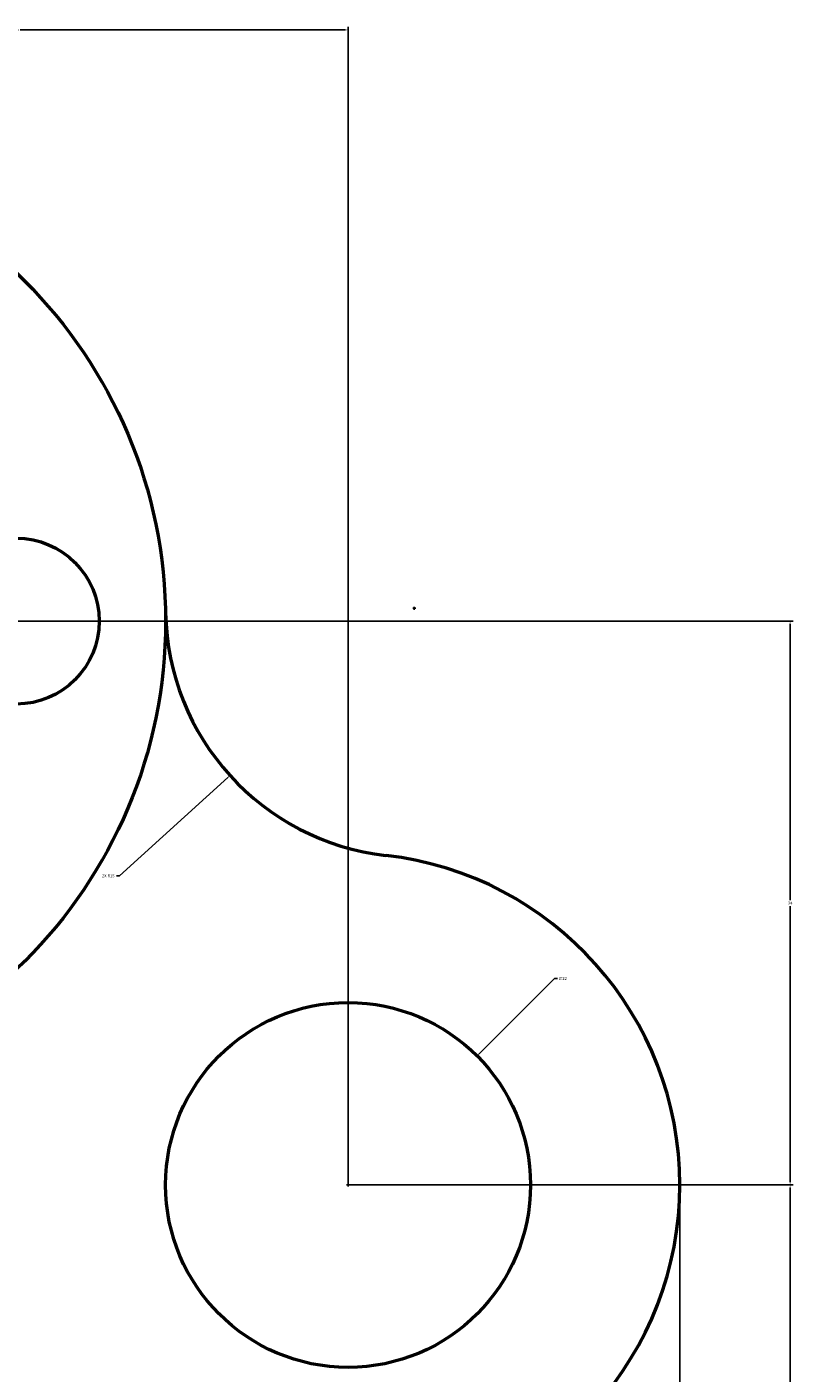
# Model space of a CAD drawing. Units: inches. Extents: x -11 to 126, y -62 to 82.
# Tile 10 of 10: x 80 to 126, y 1 to 82. Entities that reach past the tile are written whole.
import ezdxf

# ---------------------------------------------------------------- set-up
doc = ezdxf.new("R2010")
doc.units = ezdxf.units.IN
doc.header["$MEASUREMENT"] = 0
doc.layers.add('M-DIMS', color=2, linetype='Continuous', lineweight=18)
doc.layers.add('M-OUTL', color=7, linetype='Continuous', lineweight=50)
doc.styles.get("Standard").update_dxf_attribs({"font": 'arial.ttf'})
doc.dimstyles.get("Standard").update_dxf_attribs({"dimtxt": 0.18, "dimasz": 0.18, "dimexe": 0.18, "dimexo": 0.0625, "dimgap": 0.09, "dimtad": 0, "dimtih": 1, "dimtoh": 1, "dimdec": 4, "dimzin": 0, "dimdsep": 46, "dimtxsty": 'Standard', "dimcen": 0.09, "dimadec": 0, "dimazin": 0, "dimtfac": 1, "dimtdec": 4, "dimtofl": 0, "dimtmove": 0, "dimatfit": 3, "dimfxl": 1, "dimtolj": 1, "dimtzin": 0, "dimarcsym": 0})

# ---------------------------------------------------------------- blocks, each defined once
blk = doc.blocks.new('*U1')
blk.add_circle((0, 0), 5)
blk = doc.blocks.new('*U2')
at = {"layer": 'M-OUTL', "color": 0, "linetype": 'ByBlock', "lineweight": -2, "transparency": 16777216}
for p, rotation in [((73.374, 60.496), 135), ((79.232, 46.354), 90), ((73.374, 32.212), 44.99999999999998)]:
    blk.add_blockref('*U1', p, dxfattribs=dict(at, rotation=rotation))
blk = doc.blocks.new('*D5')
at = {"layer": 'Defpoints', "color": 0, "transparency": 16777216}
for p in [(119.232, 12.354), (-0.749, 11.479), (119.232, -57.296)]:
    blk.add_point(p, dxfattribs=at)
at = {"layer": 'M-DIMS', "color": 0, "lineweight": -2, "transparency": 16777216}
for p, q in [((119.232, 12.292), (119.232, -57.476)), ((-0.749, 11.416), (-0.749, -57.476)), ((-0.569, -57.296), (58.786, -57.296)), ((119.052, -57.296), (59.696, -57.296))]:
    blk.add_line(p, q, dxfattribs=at)
at = {"layer": 'M-DIMS', "color": 0, "transparency": 16777216}
for points in [[(-0.569, -57.266), (-0.569, -57.326), (-0.749, -57.296)], [(119.052, -57.266), (119.052, -57.326), (119.232, -57.296)]]:
    blk.add_solid(points, dxfattribs=at)
at = {"layer": 'M-DIMS', "color": 0, "transparency": 16777216, "insert": (59.241, -57.296), "char_height": 0.18, "attachment_point": 5}
blk.add_mtext('\\A1;119.98', dxfattribs=at)
blk = doc.blocks.new('*D8')
at = {"layer": 'Defpoints', "color": 0, "transparency": 16777216}
for p in [(99.232, 82.004), (59.232, 46.354), (99.232, 12.354)]:
    blk.add_point(p, dxfattribs=at)
at = {"layer": 'M-DIMS', "color": 0, "lineweight": -2, "transparency": 16777216}
for p, q in [((59.232, 46.417), (59.232, 82.184)), ((59.412, 82.004), (79.009, 82.004)), ((99.052, 82.004), (79.454, 82.004)), ((99.232, 12.417), (99.232, 82.184))]:
    blk.add_line(p, q, dxfattribs=at)
at = {"layer": 'M-DIMS', "color": 0, "transparency": 16777216}
for points in [[(59.412, 82.034), (59.412, 81.974), (59.232, 82.004)], [(99.052, 82.034), (99.052, 81.974), (99.232, 82.004)]]:
    blk.add_solid(points, dxfattribs=at)
at = {"layer": 'M-DIMS', "color": 0, "transparency": 16777216, "insert": (79.232, 82.004), "char_height": 0.18, "attachment_point": 5}
blk.add_mtext('\\A1;40', dxfattribs=at)
blk = doc.blocks.new('*D9')
at = {"layer": 'Defpoints', "color": 0, "transparency": 16777216}
for p in [(99.232, 12.354), (125.882, 12.354), (59.232, -21.646)]:
    blk.add_point(p, dxfattribs=at)
at = {"layer": 'M-DIMS', "color": 0, "lineweight": -2, "transparency": 16777216}
for p, q in [((99.294, 12.354), (126.062, 12.354)), ((125.882, 12.174), (125.882, -4.464)), ((125.882, -21.466), (125.882, -4.828)), ((59.294, -21.646), (126.062, -21.646))]:
    blk.add_line(p, q, dxfattribs=at)
at = {"layer": 'M-DIMS', "color": 0, "transparency": 16777216}
for points in [[(125.852, 12.174), (125.912, 12.174), (125.882, 12.354)], [(125.852, -21.466), (125.912, -21.466), (125.882, -21.646)]]:
    blk.add_solid(points, dxfattribs=at)
at = {"layer": 'M-DIMS', "color": 0, "transparency": 16777216, "insert": (125.882, -4.646), "char_height": 0.18, "attachment_point": 5}
blk.add_mtext('\\A1;34', dxfattribs=at)
blk = doc.blocks.new('*D10')
at = {"layer": 'Defpoints', "color": 0, "transparency": 16777216}
for p in [(59.232, 46.354), (125.882, 46.354), (99.232, 12.354)]:
    blk.add_point(p, dxfattribs=at)
at = {"layer": 'M-DIMS', "color": 0, "lineweight": -2, "transparency": 16777216}
for p, q in [((59.294, 46.354), (126.062, 46.354)), ((125.882, 46.174), (125.882, 29.536)), ((125.882, 12.534), (125.882, 29.172)), ((99.294, 12.354), (126.062, 12.354))]:
    blk.add_line(p, q, dxfattribs=at)
at = {"layer": 'M-DIMS', "color": 0, "transparency": 16777216}
for points in [[(125.852, 46.174), (125.912, 46.174), (125.882, 46.354)], [(125.852, 12.534), (125.912, 12.534), (125.882, 12.354)]]:
    blk.add_solid(points, dxfattribs=at)
at = {"layer": 'M-DIMS', "color": 0, "transparency": 16777216, "insert": (125.882, 29.354), "char_height": 0.18, "attachment_point": 5}
blk.add_mtext('\\A1;34', dxfattribs=at)
blk = doc.blocks.new('*D17')
at = {"layer": 'Defpoints', "color": 0, "transparency": 16777216}
for p in [(103.225, 47.126), (92.117, 37.045)]:
    blk.add_point(p, dxfattribs=at)
at = {"layer": 'M-DIMS', "color": 0, "lineweight": -2, "transparency": 16777216}
for p, q in [((103.135, 47.126), (103.315, 47.126)), ((103.225, 47.036), (103.225, 47.216)), ((85.452, 30.997), (91.984, 36.924)), ((85.272, 30.997), (85.452, 30.997))]:
    blk.add_line(p, q, dxfattribs=at)
at = {"layer": 'M-DIMS', "color": 0, "transparency": 16777216}
blk.add_solid([(91.964, 36.946), (92.004, 36.902), (92.117, 37.045)], dxfattribs=at)
at = {"layer": 'M-DIMS', "color": 0, "transparency": 16777216, "insert": (84.772, 30.997), "char_height": 0.18, "attachment_point": 5}
blk.add_mtext('\\A1;2X R15', dxfattribs=at)
blk = doc.blocks.new('*D19')
at = {"layer": 'Defpoints', "color": 0, "transparency": 16777216}
for p in [(107.006, 20.136), (91.457, 4.572)]:
    blk.add_point(p, dxfattribs=at)
at = {"layer": 'M-DIMS', "color": 0, "lineweight": -2, "transparency": 16777216}
for p, q in [((111.671, 24.805), (107.133, 20.263)), ((111.851, 24.805), (111.671, 24.805)), ((99.142, 12.354), (99.322, 12.354)), ((99.232, 12.264), (99.232, 12.444))]:
    blk.add_line(p, q, dxfattribs=at)
at = {"layer": 'M-DIMS', "color": 0, "transparency": 16777216}
blk.add_solid([(107.112, 20.285), (107.155, 20.242), (107.006, 20.136)], dxfattribs=at)
at = {"layer": 'M-DIMS', "color": 0, "transparency": 16777216, "insert": (112.167, 24.805), "char_height": 0.18, "attachment_point": 5}
blk.add_mtext('\\A1;∅22', dxfattribs=at)

msp = doc.modelspace()

# ---------------------------------------------------------------- linework, layer by layer
at = {"layer": 'M-OUTL'}
for centre, radius in [((59.232, 46.354), 29), ((99.232, 12.354), 11), ((59.232, -21.646), 29)]:
    msp.add_circle(centre, radius, dxfattribs=at)
for centre, radius, start, end in [((103.225, 47.126), 15, 181.00462, 263.44872), ((99.232, 12.354), 20, 276.55128, 83.44872)]:
    msp.add_arc(centre, radius, start, end, dxfattribs=at)

# ---------------------------------------------------------------- block references
msp.add_blockref('*U2', (0, 0), dxfattribs=at)

# ---------------------------------------------------------------- dimensions: what is measured, and where the dimension line sits
at = {"layer": 'M-DIMS'}
for base, p1, p2, override, picture, middle in [((99.232, 82.004), (59.232, 46.354), (99.232, 12.354), {"dimdec": 0, "dimlfac": 1, "dimrnd": 0, "dimzin": 0, "dimdsep": 46, "dimlunit": 2}, '*D8', (79.232, 82.004)), ((119.232, -57.296), (-0.749, 11.479), (119.232, 12.354), {"dimdec": 2, "dimlfac": 1, "dimrnd": 0, "dimzin": 0, "dimdsep": 46, "dimlunit": 2}, '*D5', (59.241, -57.296))]:
    dim = msp.add_linear_dim(base=base, p1=p1, p2=p2, dimstyle='Standard', override=override, dxfattribs=at)
    dim.commit()
    dim.dimension.update_dxf_attribs({"geometry": picture, "text_midpoint": middle})
dim = msp.add_radius_dim(center=(103.225, 47.126), mpoint=(92.117, 37.045), text='2X <>', dimstyle='Standard', override={"dimdec": 0, "dimlfac": 1, "dimrnd": 0, "dimzin": 0, "dimdsep": 46, "dimlunit": 2}, dxfattribs=at)
dim.commit()
dim.dimension.update_dxf_attribs({"geometry": '*D17', "text_midpoint": (84.772, 30.997), "dimtype": 164})
for base, p1, p2, picture, middle in [((125.882, 46.354), (99.232, 12.354), (59.232, 46.354), '*D10', (125.882, 29.354)), ((125.882, 12.354), (59.232, -21.646), (99.232, 12.354), '*D9', (125.882, -4.646))]:
    dim = msp.add_linear_dim(base=base, p1=p1, p2=p2, angle=90, dimstyle='Standard', override={"dimdec": 0, "dimlfac": 1, "dimrnd": 0, "dimzin": 0, "dimdsep": 46, "dimlunit": 2}, dxfattribs=at)
    dim.commit()
    dim.dimension.update_dxf_attribs({"geometry": picture, "text_midpoint": middle})
dim = msp.add_diameter_dim_2p(p1=(91.457, 4.572), p2=(107.006, 20.136), dimstyle='Standard', override={"dimdec": 0, "dimlfac": 1, "dimrnd": 0, "dimzin": 0, "dimdsep": 46, "dimlunit": 2}, dxfattribs=at)
dim.commit()
dim.dimension.update_dxf_attribs({"geometry": '*D19', "text_midpoint": (112.167, 24.805), "dimtype": 163})

doc.saveas('drawing.dxf')
